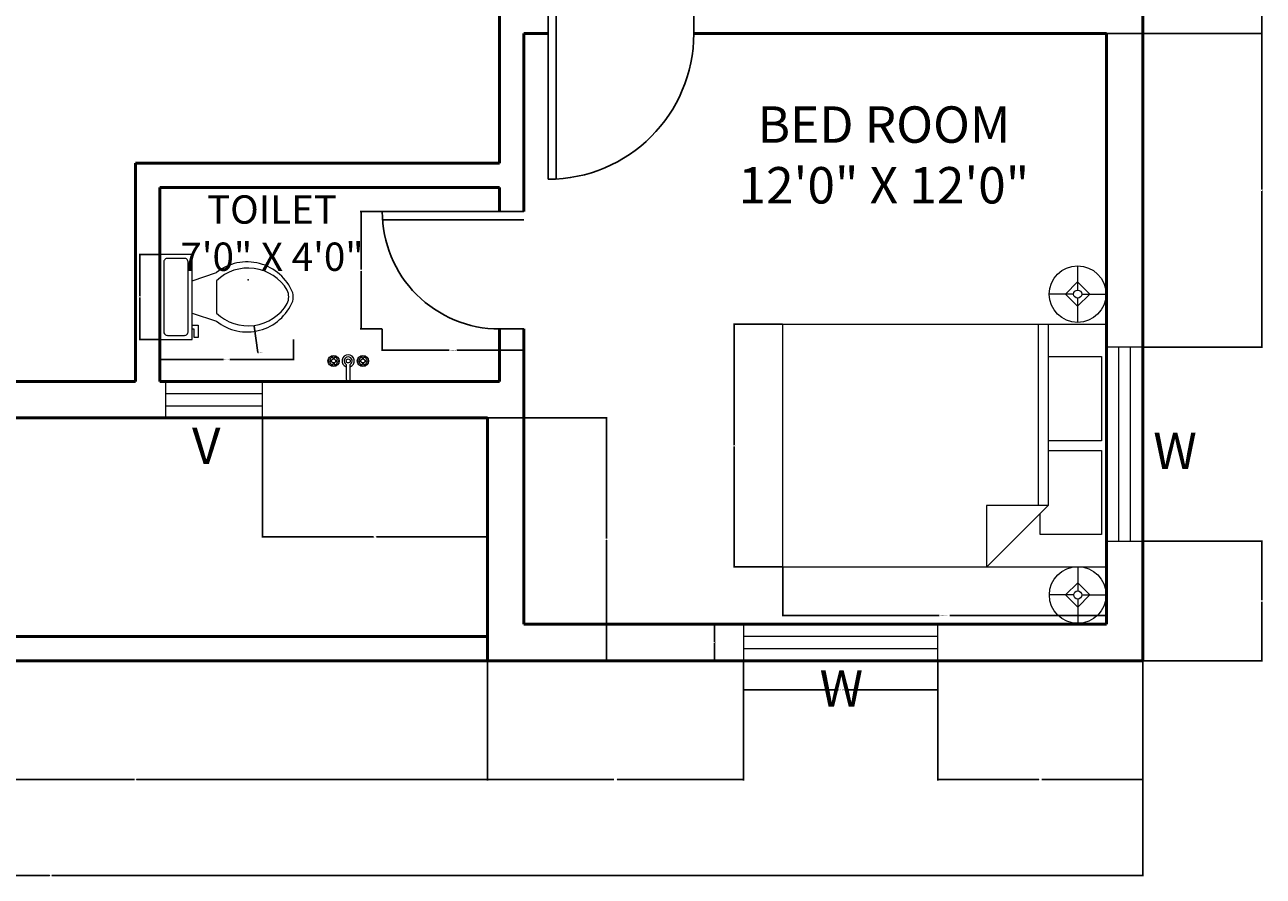
# Model space of a CAD drawing. Units: inches. Extents: x 1727 to 2326, y 1693 to 2164.
# Tile 2 of 3: x 2020 to 2326, y 1693 to 1904. Entities that reach past the tile are written whole.
import ezdxf

# ---------------------------------------------------------------- set-up
doc = ezdxf.new("R2010")
doc.units = ezdxf.units.IN
for name, color, linetype, lineweight in [('A-ANNO-DIMS', 2, 'Continuous', 18), ('A-ANNO-TEXT', 3, 'Continuous', 18), ('A-AREA-IDEN', 7, 'Continuous', 25), ('A-DOOR', 3, 'Continuous', 25), ('A-FLOR-FIXT', 9, 'Continuous', 20), ('A-FURN', 8, 'Continuous', 18), ('A-GLAZ', 4, 'Continuous', 18), ('A-WALL', 7, 'Continuous', 50)]:
    doc.layers.add(name, color=color, linetype=linetype, lineweight=lineweight)
doc.styles.add('Annotative', font='arial.ttf')
doc.styles.get("Standard").update_dxf_attribs({"font": 'arial.ttf'})
doc.dimstyles.get("Standard").update_dxf_attribs({"dimtxt": 0.18, "dimasz": 0.18, "dimexe": 0.18, "dimexo": 0.0625, "dimgap": 0.09, "dimtad": 0, "dimtih": 1, "dimtoh": 1, "dimdec": 4, "dimzin": 0, "dimdsep": 46, "dimtxsty": 'Standard', "dimcen": 0.09, "dimadec": 0, "dimazin": 0, "dimtfac": 1, "dimtdec": 4, "dimtofl": 0, "dimtmove": 0, "dimatfit": 3, "dimfxl": 1, "dimtolj": 1, "dimtzin": 0, "dimarcsym": 0})

# ---------------------------------------------------------------- blocks, each defined once
blk = doc.blocks.new('Toilet - top')
for p, q in [((9.5, -6), (9.5, -2)), ((-10, -8.5), (-8, -8.5)), ((-10, -9.5), (-10, -8.5)), ((-8, -8.5), (-8, -8)), ((-7, -8), (-7, -9.5)), ((-4, -8), (-6, -14)), ((4, -8), (6, -14)), ((-7, -9.5), (-10, -9.5)), ((4, -14), (-4, -14))]:
    blk.add_line(p, q)
blk.add_lwpolyline([(10.5, -8), (10.5, 0), (-10.5, 0), (-10.5, -8)], close=True)
for points in [[(-9.5, -2), (-9.5, -6)], [(8.5, -1), (-8.5, -1)], [(-8.5, -7), (8.5, -7)]]:
    blk.add_lwpolyline(points)
for centre, radius, start, end in [((-8.62, -1.88), 0.884, 81.8699, 188.1301), ((8.62, -1.88), 0.884, 351.8699, 98.1301), ((-8.62, -6.12), 0.884, 171.8699, 278.1301), ((8.62, -6.12), 0.884, 261.8699, 8.1301), ((3.52, -21.58), 12.17, 141.4691, 247.9714), ((4.2, -21.82), 11.33, 136.3677, 238.9468), ((-3.52, -21.58), 12.17, 292.0284, 38.5307), ((-4.2, -21.82), 11.33, 301.053, 43.6321), ((0, -27.88), 4, 245.7318, 294.2682), ((0, -29), 4, 254.8605, 285.1395)]:
    blk.add_arc(centre, radius, start, end)
blk = doc.blocks.new('Faucet - Bathroom top')
for p, q in [((-4.107, 0.125), (-4.375, 0.125)), ((-3.75, 0.4788), (-3.75, 0.75)), ((-3.5, 0.482), (-3.5, 0.75)), ((-3.1461, 0.125), (-2.875, 0.125)), ((3.143, 0.125), (2.875, 0.125)), ((3.5, 0.4788), (3.5, 0.75)), ((3.75, 0.482), (3.75, 0.75)), ((4.1039, 0.125), (4.375, 0.125)), ((-4.1039, -0.125), (-4.375, -0.125)), ((-3.75, -0.4821), (-3.75, -0.75)), ((-3.5, -0.4789), (-3.5, -0.75)), ((-3.143, -0.125), (-2.875, -0.125)), ((-0.5, -0.8639), (-0.5, -4.5)), ((0.5, -4.5), (0.5, -0.8631)), ((3.1461, -0.125), (2.875, -0.125)), ((3.5, -0.4821), (3.5, -0.75)), ((3.75, -0.4789), (3.75, -0.75)), ((4.107, -0.125), (4.375, -0.125))]:
    blk.add_line(p, q)
for centre, radius in [((-3.625, 0), 1.375), ((-4.625, 0), 0.2795), ((-3.625, 0), 0.5), ((-3.625, 1), 0.2795), ((-2.625, 0), 0.2795), ((0, 0), 0.5), ((3.625, 0), 1.375), ((2.625, 0), 0.2795), ((3.625, 0), 0.5), ((3.625, 1), 0.2795), ((4.625, 0), 0.2795), ((-3.625, -1), 0.2795), ((3.625, -1), 0.2795)]:
    blk.add_circle(centre, radius)
for centre, radius, start, end in [((-3.625, 0), 1, 105.2407, 164.2093), ((-3.625, 0), 1, 16.44125, 74.07887), ((0, 0), 1.5, 289.6514, 250.3603), ((0, 0), 1, 300.3431, 239.7554), ((3.625, 0), 1, 106.12, 164.0884), ((3.625, 0), 1, 16.23422, 73.90469), ((-3.625, 0), 1, 196.2342, 253.9047), ((-3.625, 0), 1, 286.12, 344.0884), ((3.625, 0), 1, 196.4413, 254.0789), ((3.625, 0), 1, 285.2407, 344.2093), ((0, -4.5), 0.5, 180, 0)]:
    blk.add_arc(centre, radius, start, end)
blk = doc.blocks.new('Bed - Queen')
for p, q in [((0, -80.00003), (0, 0)), ((0, 0), (59.99999, 0)), ((59.99999, 0), (59.99999, -80.00003)), ((7.99999, -1.2), (28.79998, -1.2)), ((7.99999, -14.4), (7.99999, -1.2)), ((28.79998, -1.2), (28.79998, -14.4)), ((31.19999, -1.2), (51.99999, -1.2)), ((31.19999, -14.4), (31.19999, -1.2)), ((51.99999, -1.2), (51.99999, -16.4)), ((0, -14.4), (44.8, -14.4)), ((59.99999, -29.6), (44.8, -14.4)), ((44.8, -14.4), (44.8, -29.6)), ((44.8, -16.8), (0, -16.8)), ((51.99999, -16.4), (46.79936, -16.4)), ((44.8, -29.6), (59.99999, -29.6)), ((59.99999, -80.00003), (0, -80.00003))]:
    blk.add_line(p, q)
blk = doc.blocks.new('Lamp - Table')
for p, q in [((0, 7), (0, 1)), ((-1, 0), (-7, 0)), ((0, 3), (-3, 0)), ((-3, 0), (0, -3)), ((3, 0), (0, 3)), ((0, -3), (3, 0)), ((1, 0), (7, 0)), ((0, -1), (0, -7))]:
    blk.add_line(p, q)
for radius in [7, 1]:
    blk.add_circle((0, 0), radius)
blk = doc.blocks.new('WIN-48IN')
for p, q in [((0, 48), (0, 0)), ((9, 48), (0, 48)), ((3, 48), (3, 0)), ((6, 0), (6, 48)), ((9, 0), (9, 48)), ((0, 0), (9, 0))]:
    blk.add_line(p, q)
blk = doc.blocks.new('VENT-24IN')
for p, q in [((0, 24), (0, 0)), ((9, 24), (0, 24)), ((3, 24), (3, 0)), ((6, 0), (6, 24)), ((9, 0), (9, 24)), ((0, 0), (9, 0))]:
    blk.add_line(p, q)
blk = doc.blocks.new('DOOR-SWING-36IN')
for p, q in [((0, 6), (0, 42)), ((2, 6), (2, 42)), ((0, 6), (0, 0)), ((2, 6), (2, 0)), ((36, 0), (36, 6))]:
    blk.add_line(p, q)
blk.add_arc((0, 6), 36, 0, 90)
blk = doc.blocks.new('DOOR-SWING-29IN')
for p, q in [((0, 29), (0, 35)), ((2, 29), (2, 35)), ((29, 35), (29, 29)), ((0, 29), (0, 0)), ((2, 29), (2, 0))]:
    blk.add_line(p, q)
blk.add_arc((0, 29), 29, 270, 0)
blk = doc.blocks.new('*D13')
at = {"layer": 'A-ANNO-DIMS', "color": 0, "lineweight": -2, "transparency": 16777216}
for p, q in [((2197.7, 1746.32), (2197.7, 1739)), ((2245.7, 1746.32), (2245.7, 1739)), ((2197.88, 1739.18), (2220.59, 1739.18)), ((2245.52, 1739.18), (2222.82, 1739.18))]:
    blk.add_line(p, q, dxfattribs=at)
at = {"layer": 'A-ANNO-DIMS', "color": 0, "transparency": 16777216}
for points in [[(2197.88, 1739.21), (2197.88, 1739.15), (2197.7, 1739.18)], [(2245.52, 1739.21), (2245.52, 1739.15), (2245.7, 1739.18)]]:
    blk.add_solid(points, dxfattribs=at)
at = {"layer": 'Defpoints', "color": 0, "transparency": 16777216}
for p in [(2197.7, 1746.38), (2245.7, 1746.38), (2245.7, 1739.18)]:
    blk.add_point(p, dxfattribs=at)
at = {"layer": 'A-ANNO-DIMS', "color": 0, "transparency": 16777216, "insert": (2221.7, 1739.18), "char_height": 0.18, "attachment_point": 5}
blk.add_mtext('\\A1;WINDOW 48 TYP.', dxfattribs=at)
blk = doc.blocks.new('*D14')
at = {"layer": 'A-ANNO-DIMS', "color": 0, "lineweight": -2, "transparency": 16777216}
for p, q in [((2197.64, 1755.38), (2190.32, 1755.38)), ((2190.5, 1755.2), (2190.5, 1751.06)), ((2190.5, 1746.56), (2190.5, 1750.7)), ((2197.64, 1746.38), (2190.32, 1746.38))]:
    blk.add_line(p, q, dxfattribs=at)
at = {"layer": 'A-ANNO-DIMS', "color": 0, "transparency": 16777216}
for points in [[(2190.47, 1755.2), (2190.53, 1755.2), (2190.5, 1755.38)], [(2190.47, 1746.56), (2190.53, 1746.56), (2190.5, 1746.38)]]:
    blk.add_solid(points, dxfattribs=at)
at = {"layer": 'Defpoints', "color": 0, "transparency": 16777216}
for p in [(2197.7, 1755.38), (2190.5, 1746.38), (2197.7, 1746.38)]:
    blk.add_point(p, dxfattribs=at)
at = {"layer": 'A-ANNO-DIMS', "color": 0, "transparency": 16777216, "insert": (2190.5, 1750.88), "char_height": 0.18, "attachment_point": 5}
blk.add_mtext('\\A1;9 TYP.', dxfattribs=at)
blk = doc.blocks.new('*D19')
at = {"layer": 'A-ANNO-DIMS', "color": 0, "lineweight": -2, "transparency": 16777216}
for p, q in [((2108.37, 1828.32), (2108.37, 1822.95)), ((2143.37, 1828.32), (2143.37, 1822.95)), ((2108.55, 1823.13), (2124.94, 1823.13)), ((2143.19, 1823.13), (2126.81, 1823.13))]:
    blk.add_line(p, q, dxfattribs=at)
at = {"layer": 'A-ANNO-DIMS', "color": 0, "transparency": 16777216}
for points in [[(2108.55, 1823.16), (2108.55, 1823.1), (2108.37, 1823.13)], [(2143.19, 1823.16), (2143.19, 1823.1), (2143.37, 1823.13)]]:
    blk.add_solid(points, dxfattribs=at)
at = {"layer": 'Defpoints', "color": 0, "transparency": 16777216}
for p in [(2108.37, 1828.38), (2143.37, 1828.38), (2143.37, 1823.13)]:
    blk.add_point(p, dxfattribs=at)
at = {"layer": 'A-ANNO-DIMS', "color": 0, "transparency": 16777216, "insert": (2125.87, 1823.13), "char_height": 0.18, "attachment_point": 5}
blk.add_mtext('\\A1;DOOR 35 TYP.', dxfattribs=at)
blk = doc.blocks.new('*D20')
at = {"layer": 'A-ANNO-DIMS', "color": 0, "lineweight": -2, "transparency": 16777216}
for p, q in [((2108.31, 1857.38), (2102.94, 1857.38)), ((2103.12, 1857.2), (2103.12, 1843.06)), ((2103.12, 1828.56), (2103.12, 1842.7)), ((2108.31, 1828.38), (2102.94, 1828.38))]:
    blk.add_line(p, q, dxfattribs=at)
at = {"layer": 'A-ANNO-DIMS', "color": 0, "transparency": 16777216}
for points in [[(2103.09, 1857.2), (2103.15, 1857.2), (2103.12, 1857.38)], [(2103.09, 1828.56), (2103.15, 1828.56), (2103.12, 1828.38)]]:
    blk.add_solid(points, dxfattribs=at)
at = {"layer": 'Defpoints', "color": 0, "transparency": 16777216}
for p in [(2108.37, 1857.38), (2103.12, 1828.38), (2108.37, 1828.38)]:
    blk.add_point(p, dxfattribs=at)
at = {"layer": 'A-ANNO-DIMS', "color": 0, "transparency": 16777216, "insert": (2103.12, 1842.88), "char_height": 0.18, "attachment_point": 5}
blk.add_mtext('\\A1;29 TYP.', dxfattribs=at)
blk = doc.blocks.new('*D21')
at = {"layer": 'A-ANNO-DIMS', "color": 0, "lineweight": -2, "transparency": 16777216}
for p, q in [((2207.37, 1769.48), (2207.37, 1757.37)), ((2287.37, 1769.48), (2287.37, 1757.37)), ((2207.55, 1757.55), (2246.07, 1757.55)), ((2287.19, 1757.55), (2248.68, 1757.55))]:
    blk.add_line(p, q, dxfattribs=at)
at = {"layer": 'A-ANNO-DIMS', "color": 0, "transparency": 16777216}
for points in [[(2207.55, 1757.58), (2207.55, 1757.52), (2207.37, 1757.55)], [(2287.19, 1757.58), (2287.19, 1757.52), (2287.37, 1757.55)]]:
    blk.add_solid(points, dxfattribs=at)
at = {"layer": 'Defpoints', "color": 0, "transparency": 16777216}
for p in [(2207.37, 1769.55), (2287.37, 1769.55), (2287.37, 1757.55)]:
    blk.add_point(p, dxfattribs=at)
at = {"layer": 'A-ANNO-DIMS', "color": 0, "transparency": 16777216, "insert": (2247.37, 1757.55), "char_height": 0.18, "attachment_point": 5}
blk.add_mtext('\\A1;QUEEN BED 80 TYP.', dxfattribs=at)
blk = doc.blocks.new('*D22')
at = {"layer": 'A-ANNO-DIMS', "color": 0, "lineweight": -2, "transparency": 16777216}
for p, q in [((2207.31, 1829.55), (2195.19, 1829.55)), ((2195.37, 1829.37), (2195.37, 1799.73)), ((2195.37, 1769.73), (2195.37, 1799.36)), ((2207.31, 1769.55), (2195.19, 1769.55))]:
    blk.add_line(p, q, dxfattribs=at)
at = {"layer": 'A-ANNO-DIMS', "color": 0, "transparency": 16777216}
for points in [[(2195.34, 1829.37), (2195.4, 1829.37), (2195.37, 1829.55)], [(2195.34, 1769.73), (2195.4, 1769.73), (2195.37, 1769.55)]]:
    blk.add_solid(points, dxfattribs=at)
at = {"layer": 'Defpoints', "color": 0, "transparency": 16777216}
for p in [(2207.37, 1829.55), (2195.37, 1769.55), (2207.37, 1769.55)]:
    blk.add_point(p, dxfattribs=at)
at = {"layer": 'A-ANNO-DIMS', "color": 0, "transparency": 16777216, "insert": (2195.37, 1799.55), "char_height": 0.18, "attachment_point": 5}
blk.add_mtext('\\A1;60 TYP.', dxfattribs=at)
blk = doc.blocks.new('*D23')
at = {"layer": 'A-ANNO-DIMS', "color": 0, "lineweight": -2, "transparency": 16777216}
for p, q in [((2053.37, 1825.74), (2053.37, 1820.67)), ((2086.42, 1825.74), (2086.42, 1820.67)), ((2053.55, 1820.85), (2069.12, 1820.85)), ((2086.24, 1820.85), (2070.67, 1820.85))]:
    blk.add_line(p, q, dxfattribs=at)
at = {"layer": 'A-ANNO-DIMS', "color": 0, "transparency": 16777216}
for points in [[(2053.55, 1820.88), (2053.55, 1820.82), (2053.37, 1820.85)], [(2086.24, 1820.88), (2086.24, 1820.82), (2086.42, 1820.85)]]:
    blk.add_solid(points, dxfattribs=at)
at = {"layer": 'Defpoints', "color": 0, "transparency": 16777216}
for p in [(2053.37, 1825.8), (2086.42, 1825.8), (2053.37, 1820.85)]:
    blk.add_point(p, dxfattribs=at)
at = {"layer": 'A-ANNO-DIMS', "color": 0, "transparency": 16777216, "insert": (2069.9, 1820.85), "char_height": 0.18, "attachment_point": 5}
blk.add_mtext('\\A1;WC 33 TYP.', dxfattribs=at)
blk = doc.blocks.new('*D24')
at = {"layer": 'A-ANNO-DIMS', "color": 0, "lineweight": -2, "transparency": 16777216}
for p, q in [((2053.31, 1846.8), (2048.24, 1846.8)), ((2048.42, 1846.62), (2048.42, 1836.48)), ((2048.42, 1825.98), (2048.42, 1836.12)), ((2053.31, 1825.8), (2048.24, 1825.8))]:
    blk.add_line(p, q, dxfattribs=at)
at = {"layer": 'A-ANNO-DIMS', "color": 0, "transparency": 16777216}
for points in [[(2048.39, 1846.62), (2048.45, 1846.62), (2048.42, 1846.8)], [(2048.39, 1825.98), (2048.45, 1825.98), (2048.42, 1825.8)]]:
    blk.add_solid(points, dxfattribs=at)
at = {"layer": 'Defpoints', "color": 0, "transparency": 16777216}
for p in [(2048.42, 1846.8), (2053.37, 1846.8), (2053.37, 1825.8)]:
    blk.add_point(p, dxfattribs=at)
at = {"layer": 'A-ANNO-DIMS', "color": 0, "transparency": 16777216, "insert": (2048.42, 1836.3), "char_height": 0.18, "attachment_point": 5}
blk.add_mtext('\\A1;21 TYP.', dxfattribs=at)
blk = doc.blocks.new('*D33')
at = {"layer": 'A-ANNO-DIMS', "color": 0, "lineweight": -2, "transparency": 16777216}
for p, q in [((1756.37, 1746.32), (1756.37, 1693.11)), ((2296.37, 1746.32), (2296.37, 1693.11)), ((1756.55, 1693.29), (2026.08, 1693.29)), ((2296.19, 1693.29), (2026.66, 1693.29))]:
    blk.add_line(p, q, dxfattribs=at)
at = {"layer": 'A-ANNO-DIMS', "color": 0, "transparency": 16777216}
for points in [[(1756.55, 1693.32), (1756.55, 1693.26), (1756.37, 1693.29)], [(2296.19, 1693.32), (2296.19, 1693.26), (2296.37, 1693.29)]]:
    blk.add_solid(points, dxfattribs=at)
at = {"layer": 'Defpoints', "color": 0, "transparency": 16777216}
for p in [(1756.37, 1746.38), (2296.37, 1746.38), (2296.37, 1693.29)]:
    blk.add_point(p, dxfattribs=at)
at = {"layer": 'A-ANNO-DIMS', "color": 0, "transparency": 16777216, "insert": (2026.37, 1693.29), "char_height": 0.18, "attachment_point": 5}
blk.add_mtext('\\A1;540', dxfattribs=at)
blk = doc.blocks.new('*D48')
at = {"layer": 'A-ANNO-DIMS', "color": 0, "lineweight": -2, "transparency": 16777216}
for p, q in [((2296.44, 1928.55), (2325.95, 1928.55)), ((2325.77, 1928.37), (2325.77, 1915.15)), ((2325.77, 1901.56), (2325.77, 1914.78)), ((2287.44, 1901.38), (2325.95, 1901.38))]:
    blk.add_line(p, q, dxfattribs=at)
at = {"layer": 'A-ANNO-DIMS', "color": 0, "transparency": 16777216}
for points in [[(2325.74, 1928.37), (2325.8, 1928.37), (2325.77, 1928.55)], [(2325.74, 1901.56), (2325.8, 1901.56), (2325.77, 1901.38)]]:
    blk.add_solid(points, dxfattribs=at)
at = {"layer": 'Defpoints', "color": 0, "transparency": 16777216}
for p in [(2296.37, 1928.55), (2287.37, 1901.38), (2325.77, 1901.38)]:
    blk.add_point(p, dxfattribs=at)
at = {"layer": 'A-ANNO-DIMS', "color": 0, "transparency": 16777216, "insert": (2325.77, 1914.96), "char_height": 0.18, "attachment_point": 5}
blk.add_mtext('\\A1;27.166', dxfattribs=at)
blk = doc.blocks.new('*D49')
at = {"layer": 'A-ANNO-DIMS', "color": 0, "lineweight": -2, "transparency": 16777216}
for p, q in [((2287.44, 1901.38), (2325.95, 1901.38)), ((2325.77, 1901.2), (2325.77, 1862.82)), ((2325.77, 1824.07), (2325.77, 1862.46)), ((2296.44, 1823.89), (2325.95, 1823.89))]:
    blk.add_line(p, q, dxfattribs=at)
at = {"layer": 'A-ANNO-DIMS', "color": 0, "transparency": 16777216}
for points in [[(2325.74, 1901.2), (2325.8, 1901.2), (2325.77, 1901.38)], [(2325.74, 1824.07), (2325.8, 1824.07), (2325.77, 1823.89)]]:
    blk.add_solid(points, dxfattribs=at)
at = {"layer": 'Defpoints', "color": 0, "transparency": 16777216}
for p in [(2287.37, 1901.38), (2296.37, 1823.89), (2325.77, 1823.89)]:
    blk.add_point(p, dxfattribs=at)
at = {"layer": 'A-ANNO-DIMS', "color": 0, "transparency": 16777216, "insert": (2325.77, 1862.64), "char_height": 0.18, "attachment_point": 5}
blk.add_mtext('\\A1;77.49', dxfattribs=at)
blk = doc.blocks.new('*D50')
at = {"layer": 'A-ANNO-DIMS', "color": 0, "lineweight": -2, "transparency": 16777216}
for p, q in [((2296.44, 1775.89), (2325.95, 1775.89)), ((2325.77, 1775.71), (2325.77, 1761.32)), ((2325.77, 1746.56), (2325.77, 1760.96)), ((2296.44, 1746.38), (2325.95, 1746.38))]:
    blk.add_line(p, q, dxfattribs=at)
at = {"layer": 'A-ANNO-DIMS', "color": 0, "transparency": 16777216}
for points in [[(2325.74, 1775.71), (2325.8, 1775.71), (2325.77, 1775.89)], [(2325.74, 1746.56), (2325.8, 1746.56), (2325.77, 1746.38)]]:
    blk.add_solid(points, dxfattribs=at)
at = {"layer": 'Defpoints', "color": 0, "transparency": 16777216}
for p in [(2296.37, 1775.89), (2296.37, 1746.38), (2325.77, 1746.38)]:
    blk.add_point(p, dxfattribs=at)
at = {"layer": 'A-ANNO-DIMS', "color": 0, "transparency": 16777216, "insert": (2325.77, 1761.14), "char_height": 0.18, "attachment_point": 5}
blk.add_mtext('\\A1;29.51', dxfattribs=at)
blk = doc.blocks.new('*D54')
at = {"layer": 'A-ANNO-DIMS', "color": 0, "lineweight": -2, "transparency": 16777216}
for p, q in [((2134.44, 1806.38), (2163.95, 1806.38)), ((2163.77, 1806.2), (2163.77, 1776.56)), ((2163.77, 1746.56), (2163.77, 1776.2)), ((2134.44, 1746.38), (2163.95, 1746.38))]:
    blk.add_line(p, q, dxfattribs=at)
at = {"layer": 'A-ANNO-DIMS', "color": 0, "transparency": 16777216}
for points in [[(2163.74, 1806.2), (2163.8, 1806.2), (2163.77, 1806.38)], [(2163.74, 1746.56), (2163.8, 1746.56), (2163.77, 1746.38)]]:
    blk.add_solid(points, dxfattribs=at)
at = {"layer": 'Defpoints', "color": 0, "transparency": 16777216}
for p in [(2134.37, 1806.38), (2134.37, 1746.38), (2163.77, 1746.38)]:
    blk.add_point(p, dxfattribs=at)
at = {"layer": 'A-ANNO-DIMS', "color": 0, "transparency": 16777216, "insert": (2163.77, 1776.38), "char_height": 0.18, "attachment_point": 5}
blk.add_mtext('\\A1;60', dxfattribs=at)
blk = doc.blocks.new('*D56')
at = {"layer": 'A-ANNO-DIMS', "color": 0, "lineweight": -2, "transparency": 16777216}
for p, q in [((1960.37, 1746.32), (1960.37, 1716.8)), ((2134.37, 1746.32), (2134.37, 1716.8)), ((1960.55, 1716.98), (2047.09, 1716.98)), ((2134.19, 1716.98), (2047.65, 1716.98))]:
    blk.add_line(p, q, dxfattribs=at)
at = {"layer": 'A-ANNO-DIMS', "color": 0, "transparency": 16777216}
for points in [[(1960.55, 1717.01), (1960.55, 1716.95), (1960.37, 1716.98)], [(2134.19, 1717.01), (2134.19, 1716.95), (2134.37, 1716.98)]]:
    blk.add_solid(points, dxfattribs=at)
at = {"layer": 'Defpoints', "color": 0, "transparency": 16777216}
for p in [(1960.37, 1746.38), (2134.37, 1746.38), (1960.37, 1716.98)]:
    blk.add_point(p, dxfattribs=at)
at = {"layer": 'A-ANNO-DIMS', "color": 0, "transparency": 16777216, "insert": (2047.37, 1716.98), "char_height": 0.18, "attachment_point": 5}
blk.add_mtext('\\A1;174', dxfattribs=at)
blk = doc.blocks.new('*D57')
at = {"layer": 'A-ANNO-DIMS', "color": 0, "lineweight": -2, "transparency": 16777216}
for p, q in [((2134.37, 1746.32), (2134.37, 1716.8)), ((2197.7, 1746.32), (2197.7, 1716.8)), ((2134.55, 1716.98), (2165.64, 1716.98)), ((2197.52, 1716.98), (2166.43, 1716.98))]:
    blk.add_line(p, q, dxfattribs=at)
at = {"layer": 'A-ANNO-DIMS', "color": 0, "transparency": 16777216}
for points in [[(2134.55, 1717.01), (2134.55, 1716.95), (2134.37, 1716.98)], [(2197.52, 1717.01), (2197.52, 1716.95), (2197.7, 1716.98)]]:
    blk.add_solid(points, dxfattribs=at)
at = {"layer": 'Defpoints', "color": 0, "transparency": 16777216}
for p in [(2134.37, 1746.38), (2197.7, 1746.38), (2134.37, 1716.98)]:
    blk.add_point(p, dxfattribs=at)
at = {"layer": 'A-ANNO-DIMS', "color": 0, "transparency": 16777216, "insert": (2166.04, 1716.98), "char_height": 0.18, "attachment_point": 5}
blk.add_mtext('\\A1;63.33', dxfattribs=at)
blk = doc.blocks.new('*D58')
at = {"layer": 'A-ANNO-DIMS', "color": 0, "lineweight": -2, "transparency": 16777216}
for p, q in [((2245.7, 1746.32), (2245.7, 1716.8)), ((2296.37, 1746.32), (2296.37, 1716.8)), ((2245.88, 1716.98), (2270.65, 1716.98)), ((2296.19, 1716.98), (2271.43, 1716.98))]:
    blk.add_line(p, q, dxfattribs=at)
at = {"layer": 'A-ANNO-DIMS', "color": 0, "transparency": 16777216}
for points in [[(2245.88, 1717.01), (2245.88, 1716.95), (2245.7, 1716.98)], [(2296.19, 1717.01), (2296.19, 1716.95), (2296.37, 1716.98)]]:
    blk.add_solid(points, dxfattribs=at)
at = {"layer": 'Defpoints', "color": 0, "transparency": 16777216}
for p in [(2245.7, 1746.38), (2296.37, 1746.38), (2245.7, 1716.98)]:
    blk.add_point(p, dxfattribs=at)
at = {"layer": 'A-ANNO-DIMS', "color": 0, "transparency": 16777216, "insert": (2271.04, 1716.98), "char_height": 0.18, "attachment_point": 5}
blk.add_mtext('\\A1;50.67', dxfattribs=at)
blk = doc.blocks.new('*D63')
at = {"layer": 'A-ANNO-DIMS', "color": 0, "lineweight": -2, "transparency": 16777216}
for p, q in [((2078.78, 1806.32), (2078.78, 1776.8)), ((2134.37, 1806.32), (2134.37, 1776.8)), ((2078.96, 1776.98), (2106.18, 1776.98)), ((2134.19, 1776.98), (2106.97, 1776.98))]:
    blk.add_line(p, q, dxfattribs=at)
at = {"layer": 'A-ANNO-DIMS', "color": 0, "transparency": 16777216}
for points in [[(2078.96, 1777.01), (2078.96, 1776.95), (2078.78, 1776.98)], [(2134.19, 1777.01), (2134.19, 1776.95), (2134.37, 1776.98)]]:
    blk.add_solid(points, dxfattribs=at)
at = {"layer": 'Defpoints', "color": 0, "transparency": 16777216}
for p in [(2078.78, 1806.38), (2134.37, 1806.38), (2078.78, 1776.98)]:
    blk.add_point(p, dxfattribs=at)
at = {"layer": 'A-ANNO-DIMS', "color": 0, "transparency": 16777216, "insert": (2106.58, 1776.98), "char_height": 0.18, "attachment_point": 5}
blk.add_mtext('\\A1;55.59', dxfattribs=at)
blk = doc.blocks.new('*D70')
at = {"layer": 'A-ANNO-DIMS', "color": 0, "lineweight": -2, "transparency": 16777216}
for p, q in [((2075.1, 1840.5), (2075.28, 1840.5)), ((2075.19, 1840.41), (2075.19, 1840.59)), ((2077.61, 1822.54), (2076.72, 1829.1)), ((2077.79, 1822.54), (2077.61, 1822.54))]:
    blk.add_line(p, q, dxfattribs=at)
at = {"layer": 'A-ANNO-DIMS', "color": 0, "transparency": 16777216}
blk.add_solid([(2076.75, 1829.1), (2076.69, 1829.09), (2076.7, 1829.28)], dxfattribs=at)
at = {"layer": 'Defpoints', "color": 0, "transparency": 16777216}
for p in [(2075.19, 1840.5), (2076.7, 1829.28)]:
    blk.add_point(p, dxfattribs=at)
at = {"layer": 'A-ANNO-DIMS', "color": 0, "transparency": 16777216, "insert": (2078.46, 1822.54), "char_height": 0.18, "attachment_point": 5}
blk.add_mtext('\\A1;4X R11.33', dxfattribs=at)

msp = doc.modelspace()

# ---------------------------------------------------------------- linework, layer by layer
at = {"layer": 'A-WALL'}
for p, q in [((2296.3729, 2106.3813), (2296.3729, 1746.3813)), ((2137.3729, 1907.3813), (2137.3729, 1869.3813)), ((2143.3729, 1901.3813), (2149.3729, 1901.3813)), ((2143.3729, 1901.3813), (2143.3729, 1857.3813)), ((2143.3729, 1901.3813), (2149.3729, 1901.3813)), ((2185.3729, 1901.3813), (2287.3729, 1901.3813)), ((2287.3729, 1901.3813), (2287.3729, 1755.3813)), ((2137.3729, 1869.3813), (2137.3729, 1875.3813)), ((2047.3729, 1869.3813), (2047.3729, 1815.3813)), ((2047.3729, 1869.3813), (2137.3729, 1869.3813)), ((2053.3729, 1863.3813), (2053.3729, 1815.3813)), ((2053.3729, 1863.3813), (2137.3729, 1863.3813)), ((2137.3729, 1863.3813), (2137.3729, 1857.3813)), ((2137.3729, 1863.3813), (2137.3729, 1857.3813)), ((2137.3729, 1828.3813), (2137.3729, 1815.3813)), ((2143.3729, 1828.3813), (2143.3729, 1755.3813)), ((1969.3729, 1815.3813), (2047.3729, 1815.3813)), ((2053.3729, 1815.3813), (2137.3729, 1815.3813)), ((1963.3729, 1806.3813), (2134.3729, 1806.3813)), ((2134.3729, 1806.3813), (2134.3729, 1755.3813)), ((2134.3729, 1755.3813), (2134.3729, 1746.3813)), ((2287.3729, 1755.3813), (2143.3729, 1755.3813)), ((2134.3729, 1752.3813), (1960.3729, 1752.3813)), ((2296.3729, 1746.3813), (1960.3729, 1746.3813))]:
    msp.add_line(p, q, dxfattribs=at)

# ---------------------------------------------------------------- block references
at = {"layer": 'A-DOOR', "extrusion": (0, 0, -1), "zscale": -1, "rotation": 180}
msp.add_blockref('DOOR-SWING-36IN', (-2149.373, 1907.3817), dxfattribs=at)
at = {"layer": 'A-DOOR', "rotation": 269.9999999999997}
msp.add_blockref('DOOR-SWING-29IN', (2108.3726, 1857.3812), dxfattribs=at)
at = {"layer": 'A-FLOR-FIXT', "rotation": 90}
msp.add_blockref('Toilet - top', (2053.3729, 1836.3035), dxfattribs=at)
at = {"layer": 'A-FLOR-FIXT'}
msp.add_blockref('Faucet - Bathroom top', (2099.9536, 1820.4731), dxfattribs=at)
at = {"layer": 'A-FURN'}
for p in [(2280.2703, 1836.9984), (2280.2926, 1762.6255)]:
    msp.add_blockref('Lamp - Table', p, dxfattribs=at)
at = {"layer": 'A-FURN', "rotation": 270}
msp.add_blockref('Bed - Queen', (2287.3729, 1829.5456), dxfattribs=at)
at = {"layer": 'A-GLAZ'}
msp.add_blockref('WIN-48IN', (2287.373, 1775.8945), dxfattribs=at)
for name, p, rotation in [('VENT-24IN', (2078.783, 1806.3814), 89.9999999999989), ('WIN-48IN', (2197.7051, 1755.3812), 269.9999999999986)]:
    msp.add_blockref(name, p, dxfattribs=dict(at, rotation=rotation))

# ---------------------------------------------------------------- texts
at = {"layer": 'A-ANNO-TEXT', "char_height": 9, "width": 33.967268, "attachment_point": 1, "style": 'Annotative'}
for s, insert in [('\\pxqc;V', (2047.8702, 1804.021)), ('\\pxqc;W', (2287.3729, 1802.7474)), ('\\pxqc;W', (2204.8765, 1744.0434))]:
    msp.add_mtext(s, dxfattribs=dict(at, insert=insert))
at = {"layer": 'A-AREA-IDEN', "attachment_point": 1, "style": 'Annotative'}
for s, insert, char_height, width in [('\\pxqc;BED ROOM \\P12\'0" X 12\'0"', (2167.3691, 1883.4032), 9, 130.001559), ('\\pxqc;TOILET \\P7\'0" X 4\'0"', (2057.7525, 1861.4124), 7, 46.708096)]:
    msp.add_mtext(s, dxfattribs=dict(at, insert=insert, char_height=char_height, width=width))

# ---------------------------------------------------------------- dimensions: what is measured, and where the dimension line sits
at = {"layer": 'A-ANNO-DIMS'}
for base, p1, p2, angle, override, picture, middle in [((2325.7729, 1901.3813), (2296.3729, 1928.5475), (2287.3729, 1901.3813), 90, {"dimdec": 3, "dimlfac": 1, "dimrnd": 0, "dimzin": 0, "dimdsep": 46, "dimlunit": 2}, '*D48', (2325.7729, 1914.9644)), ((2325.7729, 1823.8942), (2287.3729, 1901.3813), (2296.3729, 1823.8942), 90, {"dimdec": 2, "dimlfac": 1, "dimrnd": 0, "dimzin": 0, "dimdsep": 46, "dimlunit": 2}, '*D49', (2325.7729, 1862.6378)), ((2078.7835, 1776.9813), (2134.3729, 1806.3813), (2078.7835, 1806.3813), 180, {"dimdec": 2, "dimlfac": 1, "dimrnd": 0, "dimzin": 0, "dimdsep": 46, "dimlunit": 2}, '*D63', (2106.5782, 1776.9813)), ((2163.7729, 1746.3813), (2134.3729, 1806.3813), (2134.3729, 1746.3813), 270, {"dimdec": 0, "dimlfac": 1, "dimrnd": 0, "dimzin": 0, "dimdsep": 46, "dimlunit": 2}, '*D54', (2163.7729, 1776.3813)), ((2325.7729, 1746.3813), (2296.3729, 1775.8942), (2296.3729, 1746.3813), 90, {"dimdec": 2, "dimlfac": 1, "dimrnd": 0, "dimzin": 0, "dimdsep": 46, "dimlunit": 2}, '*D50', (2325.7729, 1761.1378)), ((1960.3729, 1716.9813), (2134.3729, 1746.3813), (1960.3729, 1746.3813), 180, {"dimdec": 0, "dimlfac": 1, "dimrnd": 0, "dimzin": 0, "dimdsep": 46, "dimlunit": 2}, '*D56', (2047.3729, 1716.9813)), ((2134.3729, 1716.9813), (2197.7049, 1746.3813), (2134.3729, 1746.3813), 180, {"dimdec": 2, "dimlfac": 1, "dimrnd": 0, "dimzin": 0, "dimdsep": 46, "dimlunit": 2}, '*D57', (2166.0389, 1716.9813)), ((2245.7049, 1716.9813), (2296.3729, 1746.3813), (2245.7049, 1746.3813), 180, {"dimdec": 2, "dimlfac": 1, "dimrnd": 0, "dimzin": 0, "dimdsep": 46, "dimlunit": 2}, '*D58', (2271.0389, 1716.9813))]:
    dim = msp.add_linear_dim(base=base, p1=p1, p2=p2, angle=angle, dimstyle='Standard', override=override, dxfattribs=at)
    dim.commit()
    dim.dimension.update_dxf_attribs({"geometry": picture, "text_midpoint": middle})
for base, p1, p2, angle, text, picture, middle in [((2103.1229, 1828.3813), (2108.3729, 1857.3813), (2108.3729, 1828.3813), 270, '<> TYP.', '*D20', (2103.1229, 1842.8813)), ((2048.4159, 1846.8035), (2053.3729, 1825.8035), (2053.3729, 1846.8035), 90, '<> TYP.', '*D24', (2048.4159, 1836.3035)), ((2195.3728, 1769.5456), (2207.3729, 1829.5456), (2207.3729, 1769.5456), 270, '<> TYP.', '*D22', (2195.3728, 1799.5456)), ((2053.3729, 1820.8465), (2086.4191, 1825.8035), (2053.3729, 1825.8035), 180, 'WC <> TYP.', '*D23', (2069.896, 1820.8465)), ((2190.5049, 1746.3813), (2197.7049, 1755.3813), (2197.7049, 1746.3813), 270, '<> TYP.', '*D14', (2190.5049, 1750.8813))]:
    dim = msp.add_linear_dim(base=base, p1=p1, p2=p2, angle=angle, text=text, dimstyle='Standard', override={"dimdec": 0, "dimlfac": 1, "dimrnd": 0, "dimzin": 0, "dimdsep": 46, "dimlunit": 2}, dxfattribs=at)
    dim.commit()
    dim.dimension.update_dxf_attribs({"geometry": picture, "text_midpoint": middle})
dim = msp.add_radius_dim(center=(2075.1903, 1840.5034), mpoint=(2076.7, 1829.2753), text='4X <>', dimstyle='Standard', override={"dimdec": 2, "dimlfac": 1, "dimrnd": 0, "dimzin": 0, "dimdsep": 46, "dimlunit": 2}, dxfattribs=at)
dim.commit()
dim.dimension.update_dxf_attribs({"geometry": '*D70', "text_midpoint": (2078.4626, 1822.5384), "dimtype": 164})
for base, p1, p2, text, picture, middle in [((2143.3729, 1823.1313), (2108.3729, 1828.3813), (2143.3729, 1828.3813), 'DOOR <> TYP.', '*D19', (2125.8729, 1823.1313)), ((2287.3729, 1757.5456), (2207.3729, 1769.5456), (2287.3729, 1769.5456), 'QUEEN BED <> TYP.', '*D21', (2247.3729, 1757.5456)), ((2245.7049, 1739.1813), (2197.7049, 1746.3813), (2245.7049, 1746.3813), 'WINDOW <> TYP.', '*D13', (2221.7049, 1739.1813))]:
    dim = msp.add_linear_dim(base=base, p1=p1, p2=p2, text=text, dimstyle='Standard', override={"dimdec": 0, "dimlfac": 1, "dimrnd": 0, "dimzin": 0, "dimdsep": 46, "dimlunit": 2}, dxfattribs=at)
    dim.commit()
    dim.dimension.update_dxf_attribs({"geometry": picture, "text_midpoint": middle})
dim = msp.add_linear_dim(base=(2296.3729, 1693.2922), p1=(1756.3729, 1746.3813), p2=(2296.3729, 1746.3813), dimstyle='Standard', override={"dimdec": 0, "dimlfac": 1, "dimrnd": 0, "dimzin": 0, "dimdsep": 46, "dimlunit": 2}, dxfattribs=at)
dim.commit()
dim.dimension.update_dxf_attribs({"geometry": '*D33', "text_midpoint": (2026.3729, 1693.2922)})

doc.saveas('drawing.dxf')
